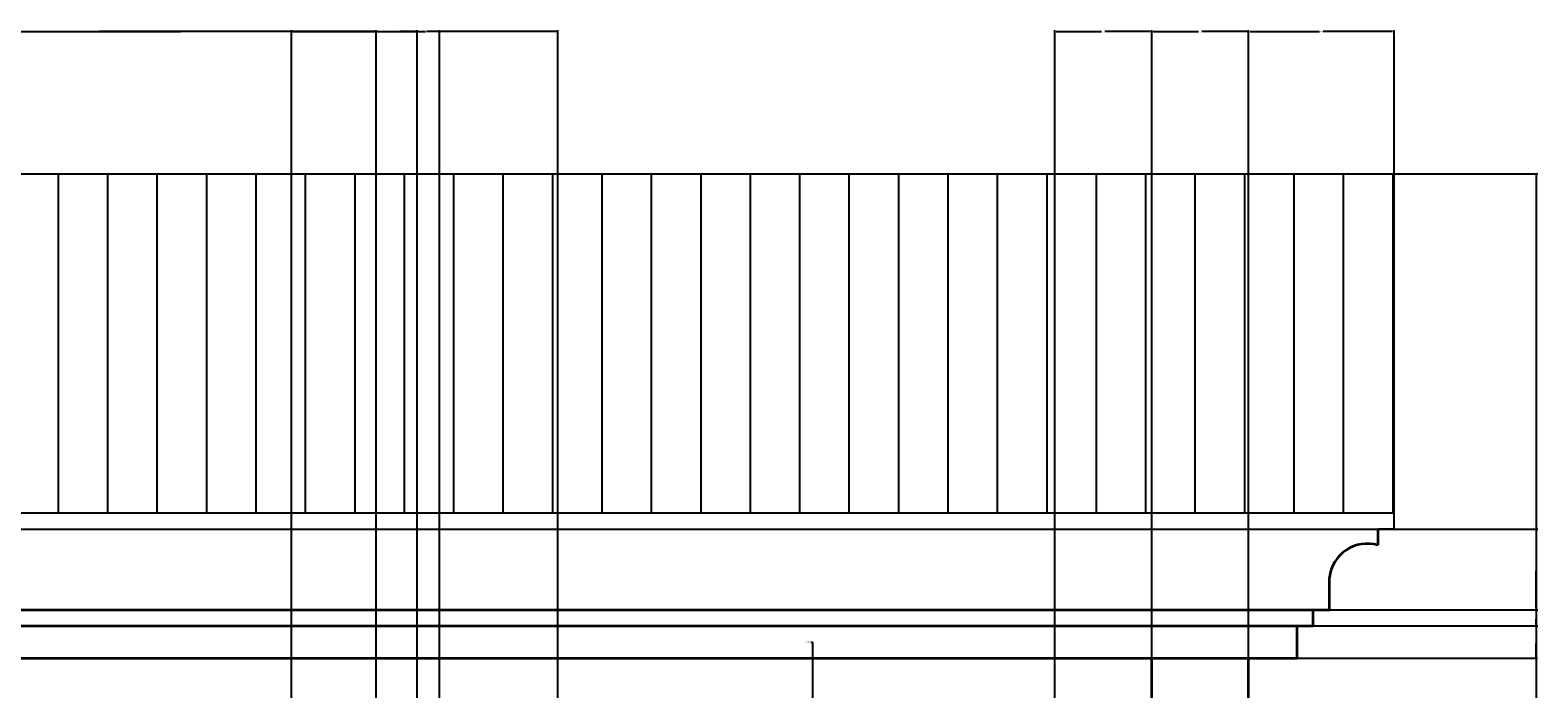
# Model space of a CAD drawing. Units: inches. Extents: x 2612 to 2948, y 481 to 865.
# Tile 7 of 7: x 2761 to 2948, y 783 to 865. Entities that reach past the tile are written whole.
import ezdxf

# ---------------------------------------------------------------- set-up
doc = ezdxf.new("R2010")
doc.units = ezdxf.units.IN
for name, color, linetype, lineweight in [('A-ANNO-DIMS', 2, 'Continuous', 18), ('A-COLS', 1, 'Continuous', 35), ('A-ELEV', 7, 'Continuous', 35), ('A-ROOF', 7, 'Continuous', 25)]:
    doc.layers.add(name, color=color, linetype=linetype, lineweight=lineweight)
doc.styles.get("Standard").update_dxf_attribs({"font": 'arial.ttf'})
doc.dimstyles.get("Standard").update_dxf_attribs({"dimtxt": 0.18, "dimasz": 0.18, "dimexe": 0.18, "dimexo": 0.0625, "dimgap": 0.09, "dimtad": 0, "dimtih": 1, "dimtoh": 1, "dimdec": 4, "dimzin": 0, "dimdsep": 46, "dimtxsty": 'Standard', "dimcen": 0.09, "dimadec": 0, "dimazin": 0, "dimtfac": 1, "dimtdec": 4, "dimtofl": 0, "dimtmove": 0, "dimatfit": 3, "dimfxl": 1, "dimtolj": 1, "dimtzin": 0, "dimarcsym": 0})

# ---------------------------------------------------------------- blocks, each defined once
blk = doc.blocks.new('*D33')
at = {"layer": 'A-ANNO-DIMS', "color": 0, "lineweight": -2, "transparency": 16777216}
for p, q in [((2756.31, 703.11), (2756.31, 864.82)), ((2756.49, 864.64), (2780.08, 864.64)), ((2804.13, 864.64), (2780.53, 864.64)), ((2804.31, 703.11), (2804.31, 864.82))]:
    blk.add_line(p, q, dxfattribs=at)
at = {"layer": 'A-ANNO-DIMS', "color": 0, "transparency": 16777216}
for points in [[(2756.49, 864.67), (2756.49, 864.61), (2756.31, 864.64)], [(2804.13, 864.67), (2804.13, 864.61), (2804.31, 864.64)]]:
    blk.add_solid(points, dxfattribs=at)
at = {"layer": 'Defpoints', "color": 0, "transparency": 16777216}
for p in [(2804.31, 864.64), (2756.31, 703.04), (2804.31, 703.04)]:
    blk.add_point(p, dxfattribs=at)
at = {"layer": 'A-ANNO-DIMS', "color": 0, "transparency": 16777216, "insert": (2780.31, 864.64), "char_height": 0.18, "attachment_point": 5}
blk.add_mtext('\\A1;48', dxfattribs=at)
blk = doc.blocks.new('*D34')
at = {"layer": 'A-ANNO-DIMS', "color": 0, "lineweight": -2, "transparency": 16777216}
for p, q in [((2804.31, 703.11), (2804.31, 864.82)), ((2804.49, 864.64), (2806.44, 864.64)), ((2809.18, 864.64), (2807.23, 864.64)), ((2809.36, 703.11), (2809.36, 864.82))]:
    blk.add_line(p, q, dxfattribs=at)
at = {"layer": 'A-ANNO-DIMS', "color": 0, "transparency": 16777216}
for points in [[(2804.49, 864.67), (2804.49, 864.61), (2804.31, 864.64)], [(2809.18, 864.67), (2809.18, 864.61), (2809.36, 864.64)]]:
    blk.add_solid(points, dxfattribs=at)
at = {"layer": 'Defpoints', "color": 0, "transparency": 16777216}
for p in [(2809.36, 864.64), (2804.31, 703.04), (2809.36, 703.04)]:
    blk.add_point(p, dxfattribs=at)
at = {"layer": 'A-ANNO-DIMS', "color": 0, "transparency": 16777216, "insert": (2806.83, 864.64), "char_height": 0.18, "attachment_point": 5}
blk.add_mtext('\\A1;5.053', dxfattribs=at)
blk = doc.blocks.new('*D35')
at = {"layer": 'A-ANNO-DIMS', "color": 0, "lineweight": -2, "transparency": 16777216}
for p, q in [((2809.36, 703.11), (2809.36, 864.82)), ((2809.54, 864.64), (2810.42, 864.64)), ((2811.95, 864.64), (2811.07, 864.64)), ((2812.13, 709.11), (2812.13, 864.82))]:
    blk.add_line(p, q, dxfattribs=at)
at = {"layer": 'A-ANNO-DIMS', "color": 0, "transparency": 16777216}
for points in [[(2809.54, 864.67), (2809.54, 864.61), (2809.36, 864.64)], [(2811.95, 864.67), (2811.95, 864.61), (2812.13, 864.64)]]:
    blk.add_solid(points, dxfattribs=at)
at = {"layer": 'Defpoints', "color": 0, "transparency": 16777216}
for p in [(2812.13, 864.64), (2812.13, 709.04), (2809.36, 703.04)]:
    blk.add_point(p, dxfattribs=at)
at = {"layer": 'A-ANNO-DIMS', "color": 0, "transparency": 16777216, "insert": (2810.75, 864.64), "char_height": 0.18, "attachment_point": 5}
blk.add_mtext('\\A1;2.77', dxfattribs=at)
blk = doc.blocks.new('*D36')
at = {"layer": 'A-ANNO-DIMS', "color": 0, "lineweight": -2, "transparency": 16777216}
for p, q in [((2888.31, 709.11), (2888.31, 864.82)), ((2888.49, 864.64), (2894.1, 864.64)), ((2900.13, 864.64), (2894.52, 864.64)), ((2900.31, 787.11), (2900.31, 864.82))]:
    blk.add_line(p, q, dxfattribs=at)
at = {"layer": 'A-ANNO-DIMS', "color": 0, "transparency": 16777216}
for points in [[(2888.49, 864.67), (2888.49, 864.61), (2888.31, 864.64)], [(2900.13, 864.67), (2900.13, 864.61), (2900.31, 864.64)]]:
    blk.add_solid(points, dxfattribs=at)
at = {"layer": 'Defpoints', "color": 0, "transparency": 16777216}
for p in [(2900.31, 864.64), (2900.31, 787.04), (2888.31, 709.04)]:
    blk.add_point(p, dxfattribs=at)
at = {"layer": 'A-ANNO-DIMS', "color": 0, "transparency": 16777216, "insert": (2894.31, 864.64), "char_height": 0.18, "attachment_point": 5}
blk.add_mtext('\\A1;12', dxfattribs=at)
blk = doc.blocks.new('*D37')
at = {"layer": 'A-ANNO-DIMS', "color": 0, "lineweight": -2, "transparency": 16777216}
for p, q in [((2900.31, 787.11), (2900.31, 864.82)), ((2900.49, 864.64), (2906.1, 864.64)), ((2912.13, 864.64), (2906.52, 864.64)), ((2912.31, 787.11), (2912.31, 864.82))]:
    blk.add_line(p, q, dxfattribs=at)
at = {"layer": 'A-ANNO-DIMS', "color": 0, "transparency": 16777216}
for points in [[(2900.49, 864.67), (2900.49, 864.61), (2900.31, 864.64)], [(2912.13, 864.67), (2912.13, 864.61), (2912.31, 864.64)]]:
    blk.add_solid(points, dxfattribs=at)
at = {"layer": 'Defpoints', "color": 0, "transparency": 16777216}
for p in [(2912.31, 864.64), (2900.31, 787.04), (2912.31, 787.04)]:
    blk.add_point(p, dxfattribs=at)
at = {"layer": 'A-ANNO-DIMS', "color": 0, "transparency": 16777216, "insert": (2906.31, 864.64), "char_height": 0.18, "attachment_point": 5}
blk.add_mtext('\\A1;12', dxfattribs=at)
blk = doc.blocks.new('*D38')
at = {"layer": 'A-ANNO-DIMS', "color": 0, "lineweight": -2, "transparency": 16777216}
for p, q in [((2912.31, 787.11), (2912.31, 864.82)), ((2912.49, 864.64), (2921.1, 864.64)), ((2930.13, 864.64), (2921.52, 864.64)), ((2930.31, 847.11), (2930.31, 864.82))]:
    blk.add_line(p, q, dxfattribs=at)
at = {"layer": 'A-ANNO-DIMS', "color": 0, "transparency": 16777216}
for points in [[(2912.49, 864.67), (2912.49, 864.61), (2912.31, 864.64)], [(2930.13, 864.67), (2930.13, 864.61), (2930.31, 864.64)]]:
    blk.add_solid(points, dxfattribs=at)
at = {"layer": 'Defpoints', "color": 0, "transparency": 16777216}
for p in [(2930.31, 864.64), (2930.31, 847.04), (2912.31, 787.04)]:
    blk.add_point(p, dxfattribs=at)
at = {"layer": 'A-ANNO-DIMS', "color": 0, "transparency": 16777216, "insert": (2921.31, 864.64), "char_height": 0.18, "attachment_point": 5}
blk.add_mtext('\\A1;18', dxfattribs=at)
blk = doc.blocks.new('*D45')
at = {"layer": 'A-ANNO-DIMS', "color": 0, "lineweight": -2, "transparency": 16777216}
for p, q in [((2640.369922, 791.044274), (2948.087422, 791.044274)), ((2947.907422, 790.864274), (2947.907422, 789.224274)), ((2947.907422, 787.224274), (2947.907422, 788.864274)), ((2642.369922, 787.044274), (2948.087422, 787.044274))]:
    blk.add_line(p, q, dxfattribs=at)
at = {"layer": 'A-ANNO-DIMS', "color": 0, "transparency": 16777216}
for points in [[(2947.877422, 790.864274), (2947.937422, 790.864274), (2947.907422, 791.044274)], [(2947.877422, 787.224274), (2947.937422, 787.224274), (2947.907422, 787.044274)]]:
    blk.add_solid(points, dxfattribs=at)
at = {"layer": 'Defpoints', "color": 0, "transparency": 16777216}
for p in [(2640.307422, 791.044274), (2947.907422, 791.044274), (2642.307422, 787.044274)]:
    blk.add_point(p, dxfattribs=at)
at = {"layer": 'A-ANNO-DIMS', "color": 0, "transparency": 16777216, "insert": (2947.907422, 789.044274), "char_height": 0.18, "attachment_point": 5}
blk.add_mtext('\\A1;4', dxfattribs=at)
blk = doc.blocks.new('*D46')
at = {"layer": 'A-ANNO-DIMS', "color": 0, "lineweight": -2, "transparency": 16777216}
for p, q in [((2638.37, 793.04), (2948.09, 793.04)), ((2947.91, 792.86), (2947.91, 792.22)), ((2947.91, 791.22), (2947.91, 791.86)), ((2640.37, 791.04), (2948.09, 791.04))]:
    blk.add_line(p, q, dxfattribs=at)
at = {"layer": 'A-ANNO-DIMS', "color": 0, "transparency": 16777216}
for points in [[(2947.88, 792.86), (2947.94, 792.86), (2947.91, 793.04)], [(2947.88, 791.22), (2947.94, 791.22), (2947.91, 791.04)]]:
    blk.add_solid(points, dxfattribs=at)
at = {"layer": 'Defpoints', "color": 0, "transparency": 16777216}
for p in [(2638.31, 793.04), (2947.91, 793.04), (2640.31, 791.04)]:
    blk.add_point(p, dxfattribs=at)
at = {"layer": 'A-ANNO-DIMS', "color": 0, "transparency": 16777216, "insert": (2947.91, 792.04), "char_height": 0.18, "attachment_point": 5}
blk.add_mtext('\\A1;2', dxfattribs=at)
blk = doc.blocks.new('*D47')
at = {"layer": 'A-ANNO-DIMS', "color": 0, "lineweight": -2, "transparency": 16777216}
for p, q in [((2632.37, 803.04), (2948.09, 803.04)), ((2947.91, 802.86), (2947.91, 798.23)), ((2947.91, 793.22), (2947.91, 797.86)), ((2638.37, 793.04), (2948.09, 793.04))]:
    blk.add_line(p, q, dxfattribs=at)
at = {"layer": 'A-ANNO-DIMS', "color": 0, "transparency": 16777216}
for points in [[(2947.88, 802.86), (2947.94, 802.86), (2947.91, 803.04)], [(2947.88, 793.22), (2947.94, 793.22), (2947.91, 793.04)]]:
    blk.add_solid(points, dxfattribs=at)
at = {"layer": 'Defpoints', "color": 0, "transparency": 16777216}
for p in [(2632.31, 803.04), (2947.91, 803.04), (2638.31, 793.04)]:
    blk.add_point(p, dxfattribs=at)
at = {"layer": 'A-ANNO-DIMS', "color": 0, "transparency": 16777216, "insert": (2947.91, 798.04), "char_height": 0.18, "attachment_point": 5}
blk.add_mtext('\\A1;10', dxfattribs=at)
blk = doc.blocks.new('*D50')
at = {"layer": 'A-ANNO-DIMS', "color": 0, "lineweight": -2, "transparency": 16777216}
for p, q in [((2745.81, 604.11), (2745.81, 864.82)), ((2745.99, 864.64), (2769.58, 864.64)), ((2793.63, 864.64), (2770.03, 864.64)), ((2793.81, 604.11), (2793.81, 864.82))]:
    blk.add_line(p, q, dxfattribs=at)
at = {"layer": 'A-ANNO-DIMS', "color": 0, "transparency": 16777216}
for points in [[(2745.99, 864.67), (2745.99, 864.61), (2745.81, 864.64)], [(2793.63, 864.67), (2793.63, 864.61), (2793.81, 864.64)]]:
    blk.add_solid(points, dxfattribs=at)
at = {"layer": 'Defpoints', "color": 0, "transparency": 16777216}
for p in [(2793.81, 864.64), (2745.81, 604.04), (2793.81, 604.04)]:
    blk.add_point(p, dxfattribs=at)
at = {"layer": 'A-ANNO-DIMS', "color": 0, "transparency": 16777216, "insert": (2769.81, 864.64), "char_height": 0.18, "attachment_point": 5}
blk.add_mtext('\\A1;48', dxfattribs=at)
blk = doc.blocks.new('*D51')
at = {"layer": 'A-ANNO-DIMS', "color": 0, "lineweight": -2, "transparency": 16777216}
for p, q in [((2793.81, 604.11), (2793.81, 864.82)), ((2793.99, 864.64), (2810.09, 864.64)), ((2826.63, 864.64), (2810.53, 864.64)), ((2826.81, 562.11), (2826.81, 864.82))]:
    blk.add_line(p, q, dxfattribs=at)
at = {"layer": 'A-ANNO-DIMS', "color": 0, "transparency": 16777216}
for points in [[(2793.99, 864.67), (2793.99, 864.61), (2793.81, 864.64)], [(2826.63, 864.67), (2826.63, 864.61), (2826.81, 864.64)]]:
    blk.add_solid(points, dxfattribs=at)
at = {"layer": 'Defpoints', "color": 0, "transparency": 16777216}
for p in [(2826.81, 864.64), (2793.81, 604.04), (2826.81, 562.04)]:
    blk.add_point(p, dxfattribs=at)
at = {"layer": 'A-ANNO-DIMS', "color": 0, "transparency": 16777216, "insert": (2810.31, 864.64), "char_height": 0.18, "attachment_point": 5}
blk.add_mtext('\\A1;33', dxfattribs=at)
blk = doc.blocks.new('*D86')
at = {"layer": 'A-ANNO-DIMS', "color": 0, "lineweight": -2, "transparency": 16777216}
for p, q in [((2930.37, 847.04), (2948.09, 847.04)), ((2947.91, 846.86), (2947.91, 673.23)), ((2947.91, 499.22), (2947.91, 672.86)), ((2930.37, 499.04), (2948.09, 499.04))]:
    blk.add_line(p, q, dxfattribs=at)
at = {"layer": 'A-ANNO-DIMS', "color": 0, "transparency": 16777216}
for points in [[(2947.88, 846.86), (2947.94, 846.86), (2947.91, 847.04)], [(2947.88, 499.22), (2947.94, 499.22), (2947.91, 499.04)]]:
    blk.add_solid(points, dxfattribs=at)
at = {"layer": 'Defpoints', "color": 0, "transparency": 16777216}
for p in [(2930.31, 847.04), (2947.91, 847.04), (2930.31, 499.04)]:
    blk.add_point(p, dxfattribs=at)
at = {"layer": 'A-ANNO-DIMS', "color": 0, "transparency": 16777216, "insert": (2947.91, 673.04), "char_height": 0.18, "attachment_point": 5}
blk.add_mtext('\\A1;348', dxfattribs=at)
blk = doc.blocks.new('*D105')
at = {"layer": 'A-ANNO-DIMS', "color": 0, "lineweight": -2, "transparency": 16777216}
for p, q in [((2858.13, 789.05), (2858.31, 789.05)), ((2858.31, 789.05), (2858.31, 763.39)), ((2858.22, 720.15), (2858.4, 720.15)), ((2858.31, 720.06), (2858.31, 720.24))]:
    blk.add_line(p, q, dxfattribs=at)
at = {"layer": 'A-ANNO-DIMS', "color": 0, "transparency": 16777216}
blk.add_solid([(2858.34, 763.39), (2858.28, 763.39), (2858.31, 763.21)], dxfattribs=at)
at = {"layer": 'Defpoints', "color": 0, "transparency": 16777216}
for p in [(2858.31, 763.21), (2858.31, 720.15)]:
    blk.add_point(p, dxfattribs=at)
at = {"layer": 'A-ANNO-DIMS', "color": 0, "transparency": 16777216, "insert": (2857.65, 789.05), "char_height": 0.18, "attachment_point": 5}
blk.add_mtext('\\A1;R43.06', dxfattribs=at)

msp = doc.modelspace()

# ---------------------------------------------------------------- linework, layer by layer
at = {"layer": 'A-COLS'}
msp.add_line((2900.3074, 703.0443), (2900.3074, 787.0443), dxfattribs=at)
at = {"layer": 'A-ELEV'}
for p, q in [((2928.3074, 803.0443), (2928.3074, 801.0443)), ((2922.3074, 793.0443), (2922.3074, 797.0443)), ((2638.3074, 793.0443), (2922.3074, 793.0443)), ((2920.3074, 791.0443), (2920.3074, 793.0443)), ((2640.3074, 791.0443), (2920.3074, 791.0443)), ((2918.3074, 787.0443), (2918.3074, 791.0443)), ((2918.3074, 791.0443), (2920.3074, 791.0443)), ((2642.3074, 787.0443), (2918.3074, 787.0443)), ((2912.3074, 703.0443), (2912.3074, 787.0443))]:
    msp.add_line(p, q, dxfattribs=at)
msp.add_arc((2926.9909, 796.519), 4.7129, 73.7794, 173.600735, dxfattribs=at)
at = {"layer": 'A-ROOF'}
for p, q in [((2630.3074, 847.0443), (2930.3074, 847.0443)), ((2764.9278, 847.0443), (2764.9278, 805.0443)), ((2771.0469, 847.0443), (2771.0469, 805.0443)), ((2777.166, 847.0443), (2777.166, 805.0443)), ((2783.2851, 847.0443), (2783.2851, 805.0443)), ((2789.4042, 847.0443), (2789.4042, 805.0443)), ((2795.5233, 847.0443), (2795.5233, 805.0443)), ((2801.6425, 847.0443), (2801.6425, 805.0443)), ((2807.7616, 847.0443), (2807.7616, 805.0443)), ((2813.8807, 847.0443), (2813.8807, 805.0443)), ((2819.9998, 847.0443), (2819.9998, 805.0443)), ((2826.1189, 847.0443), (2826.1189, 805.0443)), ((2832.238, 847.0443), (2832.238, 805.0443)), ((2838.3571, 847.0443), (2838.3571, 805.0443)), ((2844.4762, 847.0443), (2844.4762, 805.0443)), ((2850.5953, 847.0443), (2850.5953, 805.0443)), ((2856.7144, 847.0443), (2856.7144, 805.0443)), ((2862.8335, 847.0443), (2862.8335, 805.0443)), ((2868.9526, 847.0443), (2868.9526, 805.0443)), ((2875.0718, 847.0443), (2875.0718, 805.0443)), ((2881.1909, 847.0443), (2881.1909, 805.0443)), ((2887.31, 847.0443), (2887.31, 805.0443)), ((2893.4291, 847.0443), (2893.4291, 805.0443)), ((2899.5482, 847.0443), (2899.5482, 805.0443)), ((2905.6673, 847.0443), (2905.6673, 805.0443)), ((2911.7864, 847.0443), (2911.7864, 805.0443)), ((2917.9055, 847.0443), (2917.9055, 805.0443)), ((2924.0246, 847.0443), (2924.0246, 805.0443)), ((2930.1437, 847.0443), (2930.1437, 805.0443)), ((2930.3074, 803.0443), (2930.3074, 847.0443)), ((2630.3074, 805.0443), (2930.3074, 805.0443)), ((2630.3074, 803.0443), (2930.3074, 803.0443)), ((2930.3074, 803.0443), (2928.3074, 803.0443))]:
    msp.add_line(p, q, dxfattribs=at)

# ---------------------------------------------------------------- dimensions: what is measured, and where the dimension line sits
at = {"layer": 'A-ANNO-DIMS'}
for base, p1, p2, override, picture, middle in [((2793.8074, 864.6443), (2745.8074, 604.0443), (2793.8074, 604.0443), {"dimdec": 0, "dimlfac": 1, "dimrnd": 0, "dimzin": 0, "dimdsep": 46, "dimlunit": 2}, '*D50', (2769.8074, 864.6443)), ((2804.3074, 864.6443), (2756.3074, 703.0443), (2804.3074, 703.0443), {"dimdec": 0, "dimlfac": 1, "dimrnd": 0, "dimzin": 0, "dimdsep": 46, "dimlunit": 2}, '*D33', (2780.3074, 864.6443)), ((2826.8074, 864.6443), (2793.8074, 604.0443), (2826.8074, 562.0443), {"dimdec": 0, "dimlfac": 1, "dimrnd": 0, "dimzin": 0, "dimdsep": 46, "dimlunit": 2}, '*D51', (2810.3074, 864.6443)), ((2809.3601, 864.6443), (2804.3074, 703.0443), (2809.3601, 703.0443), {"dimdec": 3, "dimlfac": 1, "dimrnd": 0, "dimzin": 0, "dimdsep": 46, "dimlunit": 2}, '*D34', (2806.8337, 864.6443)), ((2812.1304, 864.6443), (2809.3601, 703.0443), (2812.1304, 709.0443), {"dimdec": 2, "dimlfac": 1, "dimrnd": 0, "dimzin": 0, "dimdsep": 46, "dimlunit": 2}, '*D35', (2810.7452, 864.6443)), ((2900.3074, 864.6443), (2888.3074, 709.0443), (2900.3074, 787.0443), {"dimdec": 0, "dimlfac": 1, "dimrnd": 0, "dimzin": 0, "dimdsep": 46, "dimlunit": 2}, '*D36', (2894.3074, 864.6443)), ((2912.3074, 864.6443), (2900.3074, 787.0443), (2912.3074, 787.0443), {"dimdec": 0, "dimlfac": 1, "dimrnd": 0, "dimzin": 0, "dimdsep": 46, "dimlunit": 2}, '*D37', (2906.3074, 864.6443)), ((2930.3074, 864.6443), (2912.3074, 787.0443), (2930.3074, 847.0443), {"dimdec": 0, "dimlfac": 1, "dimrnd": 0, "dimzin": 0, "dimdsep": 46, "dimlunit": 2}, '*D38', (2921.3074, 864.6443))]:
    dim = msp.add_linear_dim(base=base, p1=p1, p2=p2, dimstyle='Standard', override=override, dxfattribs=at)
    dim.commit()
    dim.dimension.update_dxf_attribs({"geometry": picture, "text_midpoint": middle})
for base, p1, p2, picture, middle in [((2947.9074, 847.0443), (2930.3074, 499.0443), (2930.3074, 847.0443), '*D86', (2947.9074, 673.0443)), ((2947.9074, 803.0443), (2638.3074, 793.0443), (2632.3074, 803.0443), '*D47', (2947.9074, 798.0443)), ((2947.9074, 793.0443), (2640.3074, 791.0443), (2638.3074, 793.0443), '*D46', (2947.9074, 792.0443)), ((2947.9074, 791.0443), (2642.3074, 787.0443), (2640.3074, 791.0443), '*D45', (2947.9074, 789.0443))]:
    dim = msp.add_linear_dim(base=base, p1=p1, p2=p2, angle=90, dimstyle='Standard', override={"dimdec": 0, "dimlfac": 1, "dimrnd": 0, "dimzin": 0, "dimdsep": 46, "dimlunit": 2}, dxfattribs=at)
    dim.commit()
    dim.dimension.update_dxf_attribs({"geometry": picture, "text_midpoint": middle})
dim = msp.add_radius_dim(center=(2858.3074, 720.1526), mpoint=(2858.307, 763.2141), dimstyle='Standard', override={"dimdec": 2, "dimlfac": 1, "dimrnd": 0, "dimzin": 0, "dimdsep": 46, "dimlunit": 2}, dxfattribs=at)
dim.commit()
dim.dimension.update_dxf_attribs({"geometry": '*D105', "text_midpoint": (2857.647, 789.0511), "dimtype": 164})

doc.saveas('drawing.dxf')
